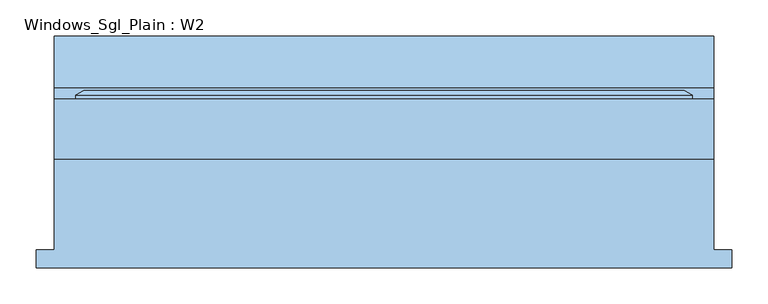
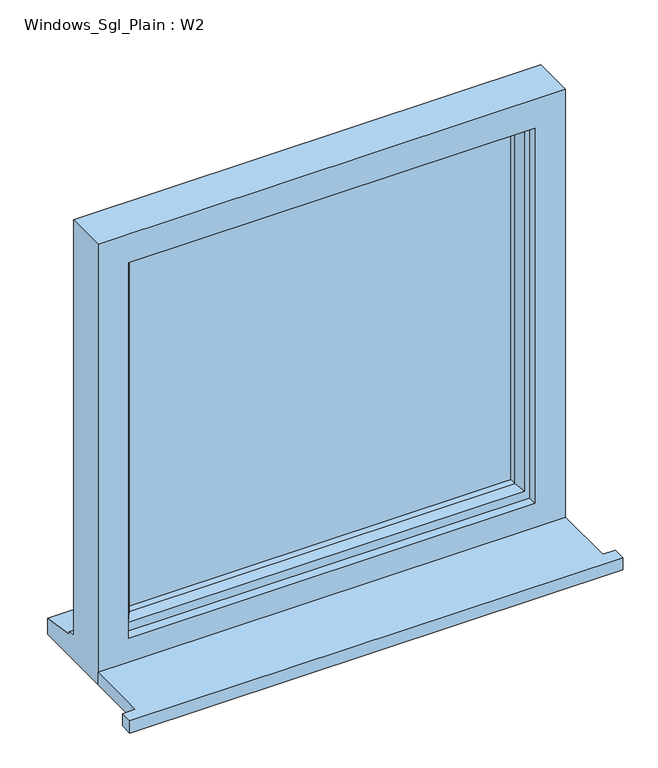
"""IFC4 building model written with IfcOpenShell, lengths in millimetres: window geometry, Windows_Sgl_Plain : W2."""

from ifc_helpers import new_model, si_unit, frame, origin, place, context, project, spatial, polyline, outline, extrude, faceted_brep, source, transform, mapped, element, save


def windows_sgl_plain_w2_7fc3d610(model_context):
    return source(origin(), model_context, "Body", "SolidModel", [
        extrude(outline(polyline([(-482.2, -146.0834322), (-482.2, -121.0834322), (-457.2, -121.0834322), (-457.2, 4.9965678), (457.2, 4.9965678), (457.2, -121.0834322), (482.2, -121.0834322), (482.2, -146.0834322), (-482.2, -146.0834322)])), frame((0.0, 0.0, 1200.0), z_axis=(0.0, 0.0, 1.0), x_axis=(1.0, 0.0, 0.0)), (0.0, 0.0, 1.0), 25.0),
        faceted_brep([(-457.2, 4.9965678, 1200.0), (457.2, 4.9965678, 1200.0), (457.2, 4.9965678, 2110.0), (-457.2, 4.9965678, 2110.0), (-397.2, 4.9965678, 2050.0), (397.2, 4.9965678, 2050.0), (397.2, 4.9965678, 1275.0), (-397.2, 4.9965678, 1275.0), (-457.2, 87.9965678, 2110.0), (-457.2, 87.9965678, 1251.0), (-457.2, 102.9965678, 1249.68767), (-457.2, 102.9965678, 1244.7449676), (-457.2, 175.4965678, 1233.8088847), (-457.2, 175.4965678, 1200.0), (457.2, 87.9965678, 2110.0), (457.2, 87.9965678, 1251.0), (-417.2, 87.9965678, 2070.0), (-417.2, 87.9965678, 1263.0), (417.2, 87.9965678, 1263.0), (417.2, 87.9965678, 2070.0), (-417.2, 22.9965678, 2070.0), (-417.2, 22.9965678, 1263.0), (417.2, 22.9965678, 2070.0), (417.2, 22.9965678, 1263.0), (-397.2, 22.9965678, 2050.0), (-397.2, 22.9965678, 1275.0), (397.2, 22.9965678, 1275.0), (397.2, 22.9965678, 2050.0), (457.2, 175.4965678, 1200.0), (457.2, 175.4965678, 1233.8088847), (457.2, 102.9965678, 1244.7449676), (457.2, 102.9965678, 1249.68767)], [[[0, 1, 2, 3], [4, 5, 6, 7]], [[0, 3, 8, 9, 10, 11, 12, 13]], [[9, 8, 14, 15], [16, 17, 18, 19]], [[17, 16, 20, 21]], [[20, 22, 23, 21], [24, 25, 26, 27]], [[24, 4, 7, 25]], [[3, 2, 14, 8]], [[16, 19, 22, 20]], [[5, 4, 24, 27]], [[15, 14, 2, 1, 28, 29, 30, 31]], [[19, 18, 23, 22]], [[5, 27, 26, 6]], [[28, 1, 0, 13]], [[29, 28, 13, 12]], [[30, 29, 12, 11]], [[31, 30, 11, 10]], [[15, 31, 10, 9]], [[21, 23, 18, 17]], [[7, 6, 26, 25]]]),
        extrude(outline(polyline([(387.2, 51.9965678), (-387.2, 51.9965678), (-387.2, 75.9965678), (387.2, 75.9965678), (387.2, 51.9965678)])), frame((0.0, 0.0, 1293.0), z_axis=(0.0, 0.0, 1.0), x_axis=(1.0, 0.0, 0.0)), (0.0, 0.0, 1.0), 747.0),
        faceted_brep([(-427.2, 87.9965678, 2080.0), (-427.2, 93.7700705, 2080.0), (-427.2, 93.7700705, 1253.0), (-427.2, 87.9965678, 1253.0), (-417.2, 22.9965678, 2070.0), (-417.2, 87.9965678, 2070.0), (-417.2, 87.9965678, 1263.0), (-417.2, 22.9965678, 1263.0), (-377.2, 37.4894677, 2030.0), (-387.3480377, 22.9965678, 2040.1480377), (-387.3480377, 22.9965678, 1292.8519623), (-377.2, 37.4894677, 1303.0), (-377.2, 51.9965678, 2030.0), (-377.2, 51.9965678, 1303.0), (-387.2, 75.9965678, 2040.0), (-387.2, 51.9965678, 2040.0), (-387.2, 51.9965678, 1293.0), (-387.2, 75.9965678, 1293.0), (-377.2, 93.7700705, 2030.0), (-377.2, 75.9965678, 2030.0), (-377.2, 75.9965678, 1303.0), (-377.2, 93.7700705, 1303.0), (-394.6457548, 99.5435732, 2047.4457548), (-394.6457548, 99.5435732, 1285.5542452), (-416.4153903, 99.5435732, 2069.2153903), (-416.4153903, 99.5435732, 1263.7846097), (427.2, 93.7700705, 1253.0), (427.2, 87.9965678, 1253.0), (417.2, 87.9965678, 1263.0), (417.2, 22.9965678, 1263.0), (387.3480377, 22.9965678, 1292.8519623), (377.2, 37.4894677, 1303.0), (377.2, 51.9965678, 1303.0), (387.2, 51.9965678, 1293.0), (387.2, 75.9965678, 1293.0), (377.2, 75.9965678, 1303.0), (377.2, 93.7700705, 1303.0), (394.6457548, 99.5435732, 1285.5542452), (416.4153903, 99.5435732, 1263.7846097), (427.2, 93.7700705, 2080.0), (427.2, 87.9965678, 2080.0), (417.2, 87.9965678, 2070.0), (417.2, 22.9965678, 2070.0), (387.3480377, 22.9965678, 2040.1480377), (377.2, 37.4894677, 2030.0), (377.2, 51.9965678, 2030.0), (387.2, 51.9965678, 2040.0), (387.2, 75.9965678, 2040.0), (377.2, 75.9965678, 2030.0), (377.2, 93.7700705, 2030.0), (394.6457548, 99.5435732, 2047.4457548), (416.4153903, 99.5435732, 2069.2153903)], [[[0, 1, 2, 3]], [[4, 5, 6, 7]], [[8, 9, 10, 11]], [[12, 8, 11, 13]], [[14, 15, 16, 17]], [[18, 19, 20, 21]], [[22, 18, 21, 23]], [[1, 24, 25, 2]], [[3, 2, 26, 27]], [[7, 6, 28, 29]], [[11, 10, 30, 31]], [[13, 11, 31, 32]], [[17, 16, 33, 34]], [[21, 20, 35, 36]], [[23, 21, 36, 37]], [[2, 25, 38, 26]], [[27, 26, 39, 40]], [[29, 28, 41, 42]], [[31, 30, 43, 44]], [[32, 31, 44, 45]], [[34, 33, 46, 47]], [[36, 35, 48, 49]], [[37, 36, 49, 50]], [[26, 38, 51, 39]], [[40, 39, 1, 0]], [[3, 27, 40, 0], [5, 41, 28, 6]], [[42, 41, 5, 4]], [[7, 29, 42, 4], [9, 43, 30, 10]], [[44, 43, 9, 8]], [[45, 44, 8, 12]], [[15, 46, 33, 16], [13, 32, 45, 12]], [[47, 46, 15, 14]], [[17, 34, 47, 14], [19, 48, 35, 20]], [[49, 48, 19, 18]], [[50, 49, 18, 22]], [[24, 51, 38, 25], [23, 37, 50, 22]], [[39, 51, 24, 1]]]),
    ])


if __name__ == "__main__":
    model = new_model("IFC4")
    model_context = context("Model", 3, world=origin())
    ifc_project = project(units=[si_unit("LENGTHUNIT", "METRE", prefix="MILLI")], contexts=[model_context])
    site = spatial("IfcSite", under=ifc_project)
    building = spatial("IfcBuilding", under=site)
    placement = place(None, origin())
    windows_sgl_plain_w2_shape = windows_sgl_plain_w2_7fc3d610(model_context)
    element("IfcWindow", 1, ObjectType="Windows_Sgl_Plain : W2", at=placement, inside=building, context=model_context, shape_type="MappedRepresentation", body=[
        mapped(windows_sgl_plain_w2_shape, transform((0.0, 0.0, 0.0), x_axis=(1.0, 0.0, 0.0), y_axis=(0.0, 1.0, 0.0), z_axis=(0.0, 0.0, 1.0))),
    ])
    save(model, "model.ifc")

# Revit data of these elements
# Type "Windows_Sgl_Plain : W2"
#   Type Mark = "57"
#   Operation = "SinglePanel"
#   Construction Type Id = "SGL"
#   Manufacturer = "Revit"
#   Keynote = "L10"
#   Analytic Construction = "Large single-glazed windows"
#   Wrap Layers (Ext) from Ext = 0.336286 ft
#   Wrap Layers (Int) from Ext = 0.582349 ft
#   Window Board Projection = 0.082021 ft
#   Window Board Extension = 0.082021 ft
#   Visual Light Transmittance = 0.9
#   Solar Heat Gain Coefficient = 0.86
#   Rough Width = 3.0 ft
#   Rough Height = 2.985564 ft
#   Height = 2.985564 ft
#   Width = 3.0 ft
#   Heat Transfer Coefficient (U) = 5.5617 W/(m²·K)
#   Glazing Thickness = 0.07874 ft
#   FrameOffset - External = 0.164042 ft
#   Frame Depth = 0.213255 ft
#   Default Head Height = 6.922572 ft
#   Cill Depth = 0.287073 ft
#   Cavity Closer Width = 0.164042 ft
#   Cavity Closer Offset from Ext = 0.336286 ft
#   Cavity Closer Depth = 0.278871 ft
#   Vis - Cavity Closers = yes
#   Define Thermal Properties by = 1
#   Material Trim = Window Frame
#   Material Glass = Glass
#   Material Frame = Window Frame
#   Wall Closure = (empty or 0)
# Element 1 (IfcWindow, "Windows_Sgl_Plain : W2")
#   Materials on its faces: "Window Frame", "Glass"
# Materials
#   "Window Frame": colour RGB 249 249 249, transparency 0, Keynote = "L10", Cost = 0
#   "Glass": class "Glass", colour RGB 0 128 192, transparency 0.9, Description = "Soda Lime Glass", Cost = 0
